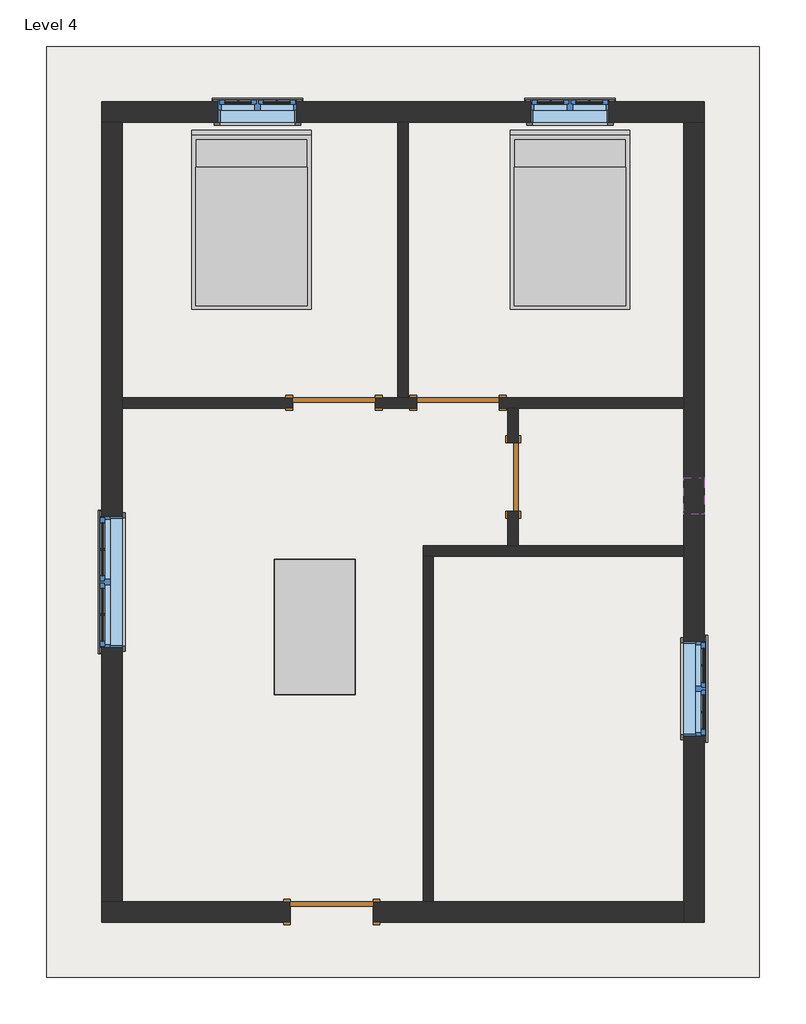
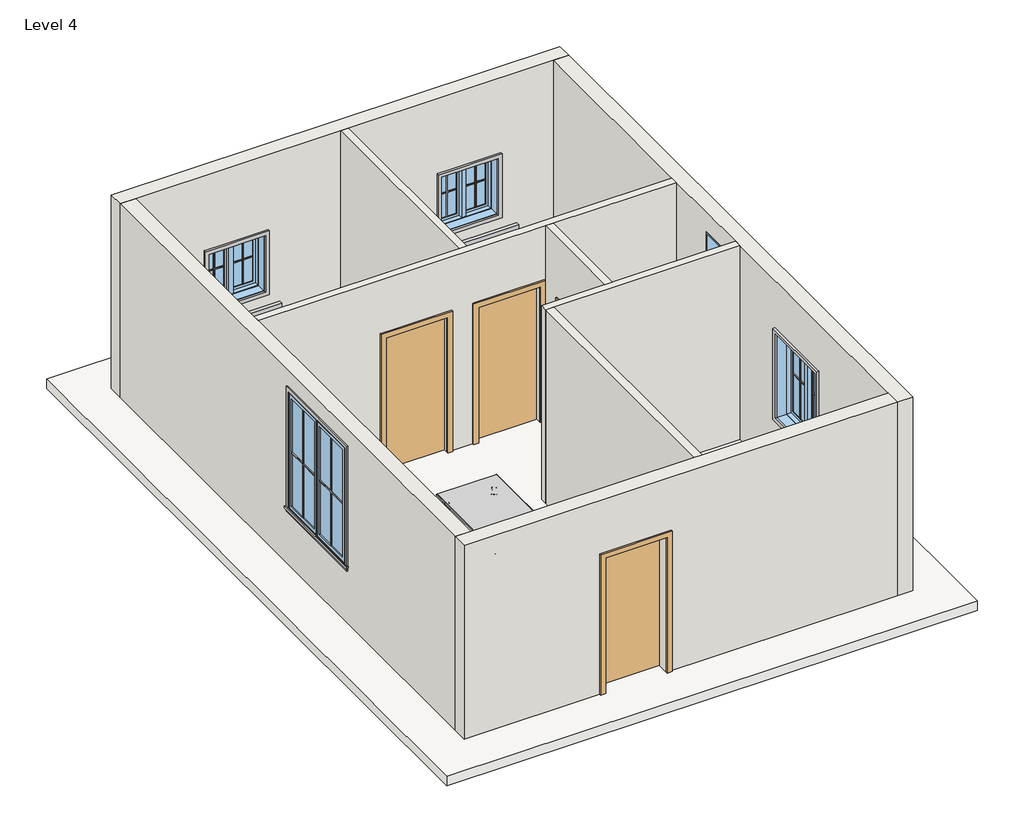
# One storey, incomplete: 16 proxies, 9 walls, 5 windows, 4 doors, 3 furniture elements, 1 roof.
"""IFC4 building model written with IfcOpenShell, lengths in millimetres."""

from ifc_helpers import new_model, si_unit, frame, origin, place, context, project, spatial, polyline, outline, extrude, faceted_brep, transform, mapped, element, save
from components import muntin_pattern_2x2_muntin_pattern_2x2_b3fe6957, muntin_pattern_2x2_muntin_pattern_2x2_3e0ecaf2, muntin_pattern_2x2_muntin_pattern_2x2_bff912c5, muntin_pattern_2x2_muntin_pattern_2x2_c2194282, muntin_pattern_2x2_muntin_pattern_2x2_88bf7f41, muntin_pattern_2x2_muntin_pattern_2x2_3dfd0a47, trim_window_exterior_flat_with_sill_41619996, trim_window_exterior_flat_with_sill_e04b3088, trim_window_exterior_flat_with_sill_4930676f, trim_window_interior_flat_picture_frame_51c85655, trim_window_interior_flat_picture_frame_2a7685fe, trim_window_interior_flat_picture_frame_dd064338, door_f2b275c1, door_e5f9f3c4, door_305aa2a5, door_0ca8825f, bed_17739_bed_17739_15c61121, dining_table_14755_dining_table_14755_d89cb775, window_aa618e30, window_339605e1, window_c95ebb39, window_9ac97e1a

model = new_model("IFC4")

# Units and contexts
model_context = context("Model", 3, world=origin())
ifc_project = project(units=[si_unit("LENGTHUNIT", "METRE", prefix="MILLI")], contexts=[model_context])

# Site, building, storey
site = spatial("IfcSite", under=ifc_project)
building = spatial("IfcBuilding", under=site)
storey = spatial("IfcBuildingStorey", under=building, Name="Level 4", Elevation=6400.8)

# Proxies
placement = place(None, origin())
muntin_pattern_2x2_muntin_pattern_2x2_shape = muntin_pattern_2x2_muntin_pattern_2x2_b3fe6957(model_context)
element("IfcBuildingElementProxy", 1, Name="Muntin Pattern_2x2 : Muntin Pattern_2x2", ObjectType="Muntin Pattern_2x2 : Muntin Pattern_2x2", at=placement, inside=storey, context=model_context, shape_type="MappedRepresentation", body=[
    mapped(muntin_pattern_2x2_muntin_pattern_2x2_shape, transform((-3079.2790084, 5068.9185985, 7385.05), x_axis=(1.0, 0.0, 0.0), y_axis=(0.0, 1.0, 0.0), z_axis=(0.0, 0.0, 1.0))),
])
element("IfcBuildingElementProxy", 2, Name="Muntin Pattern_2x2 : Muntin Pattern_2x2", ObjectType="Muntin Pattern_2x2 : Muntin Pattern_2x2", at=placement, inside=storey, context=model_context, shape_type="MappedRepresentation", body=[
    mapped(muntin_pattern_2x2_muntin_pattern_2x2_shape, transform((378.2959916, 5068.9185985, 7385.05), x_axis=(1.0, 0.0, 0.0), y_axis=(0.0, 1.0, 0.0), z_axis=(0.0, 0.0, 1.0))),
])
muntin_pattern_2x2_muntin_pattern_2x2_2_shape = muntin_pattern_2x2_muntin_pattern_2x2_3e0ecaf2(model_context)
element("IfcBuildingElementProxy", 3, Name="Muntin Pattern_2x2 : Muntin Pattern_2x2", ObjectType="Muntin Pattern_2x2 : Muntin Pattern_2x2", at=placement, inside=storey, context=model_context, shape_type="MappedRepresentation", body=[
    mapped(muntin_pattern_2x2_muntin_pattern_2x2_2_shape, transform((-2650.6540084, 5068.9185985, 7385.05), x_axis=(-1.0, 0.0, 0.0), y_axis=(0.0, -1.0, 0.0), z_axis=(0.0, 0.0, 1.0))),
])
element("IfcBuildingElementProxy", 4, Name="Muntin Pattern_2x2 : Muntin Pattern_2x2", ObjectType="Muntin Pattern_2x2 : Muntin Pattern_2x2", at=placement, inside=storey, context=model_context, shape_type="MappedRepresentation", body=[
    mapped(muntin_pattern_2x2_muntin_pattern_2x2_2_shape, transform((806.9209916, 5068.9185985, 7385.05), x_axis=(-1.0, 0.0, 0.0), y_axis=(0.0, -1.0, 0.0), z_axis=(0.0, 0.0, 1.0))),
])
muntin_pattern_2x2_muntin_pattern_2x2_3_shape = muntin_pattern_2x2_muntin_pattern_2x2_bff912c5(model_context)
element("IfcBuildingElementProxy", 5, Name="Muntin Pattern_2x2 : Muntin Pattern_2x2", ObjectType="Muntin Pattern_2x2 : Muntin Pattern_2x2", at=placement, inside=storey, context=model_context, shape_type="MappedRepresentation", body=[
    mapped(muntin_pattern_2x2_muntin_pattern_2x2_3_shape, transform((-4579.4665084, -596.8689015, 7385.05), x_axis=(0.0, 1.0, 0.0), y_axis=(-1.0, 0.0, 0.0), z_axis=(0.0, 0.0, 1.0))),
])
muntin_pattern_2x2_muntin_pattern_2x2_4_shape = muntin_pattern_2x2_muntin_pattern_2x2_c2194282(model_context)
element("IfcBuildingElementProxy", 6, Name="Muntin Pattern_2x2 : Muntin Pattern_2x2", ObjectType="Muntin Pattern_2x2 : Muntin Pattern_2x2", at=placement, inside=storey, context=model_context, shape_type="MappedRepresentation", body=[
    mapped(muntin_pattern_2x2_muntin_pattern_2x2_4_shape, transform((-4579.4665084, 123.8560985, 7385.05), x_axis=(0.0, -1.0, 0.0), y_axis=(1.0, 0.0, 0.0), z_axis=(0.0, 0.0, 1.0))),
])
muntin_pattern_2x2_muntin_pattern_2x2_5_shape = muntin_pattern_2x2_muntin_pattern_2x2_88bf7f41(model_context)
element("IfcBuildingElementProxy", 7, Name="Muntin Pattern_2x2 : Muntin Pattern_2x2", ObjectType="Muntin Pattern_2x2 : Muntin Pattern_2x2", at=placement, inside=storey, context=model_context, shape_type="MappedRepresentation", body=[
    mapped(muntin_pattern_2x2_muntin_pattern_2x2_5_shape, transform((2068.9834916, -1158.8439015, 7385.05), x_axis=(0.0, -1.0, 0.0), y_axis=(1.0, 0.0, 0.0), z_axis=(0.0, 0.0, 1.0))),
])
muntin_pattern_2x2_muntin_pattern_2x2_6_shape = muntin_pattern_2x2_muntin_pattern_2x2_3dfd0a47(model_context)
element("IfcBuildingElementProxy", 8, Name="Muntin Pattern_2x2 : Muntin Pattern_2x2", ObjectType="Muntin Pattern_2x2 : Muntin Pattern_2x2", at=placement, inside=storey, context=model_context, shape_type="MappedRepresentation", body=[
    mapped(muntin_pattern_2x2_muntin_pattern_2x2_6_shape, transform((2068.9834916, -1676.3689015, 7385.05), x_axis=(0.0, 1.0, 0.0), y_axis=(-1.0, 0.0, 0.0), z_axis=(0.0, 0.0, 1.0))),
])
trim_window_exterior_flat_with_sill_shape = trim_window_exterior_flat_with_sill_41619996(model_context)
element("IfcBuildingElementProxy", 9, Name="Trim-Window-Exterior-Flat : with Sill", ObjectType="Trim-Window-Exterior-Flat : with Sill", at=placement, inside=storey, context=model_context, shape_type="MappedRepresentation", body=[
    mapped(trim_window_exterior_flat_with_sill_shape, transform((-2864.9665084, 5078.4435985, 8229.6), x_axis=(-1.0, 0.0, 0.0), y_axis=(0.0, 0.0, 1.0), z_axis=(0.0, 1.0, 0.0))),
])
element("IfcBuildingElementProxy", 10, Name="Trim-Window-Exterior-Flat : with Sill", ObjectType="Trim-Window-Exterior-Flat : with Sill", at=placement, inside=storey, context=model_context, shape_type="MappedRepresentation", body=[
    mapped(trim_window_exterior_flat_with_sill_shape, transform((592.6084916, 5078.4435985, 8229.6), x_axis=(-1.0, 0.0, 0.0), y_axis=(0.0, 0.0, 1.0), z_axis=(0.0, 1.0, 0.0))),
])
trim_window_exterior_flat_with_sill_2_shape = trim_window_exterior_flat_with_sill_e04b3088(model_context)
element("IfcBuildingElementProxy", 11, Name="Trim-Window-Exterior-Flat : with Sill", ObjectType="Trim-Window-Exterior-Flat : with Sill", at=placement, inside=storey, context=model_context, shape_type="MappedRepresentation", body=[
    mapped(trim_window_exterior_flat_with_sill_2_shape, transform((-4588.9915084, -236.5064015, 9144.0), x_axis=(0.0, -1.0, 0.0), y_axis=(0.0, 0.0, 1.0), z_axis=(-1.0, 0.0, 0.0))),
])
trim_window_exterior_flat_with_sill_3_shape = trim_window_exterior_flat_with_sill_4930676f(model_context)
element("IfcBuildingElementProxy", 12, Name="Trim-Window-Exterior-Flat : with Sill", ObjectType="Trim-Window-Exterior-Flat : with Sill", at=placement, inside=storey, context=model_context, shape_type="MappedRepresentation", body=[
    mapped(trim_window_exterior_flat_with_sill_3_shape, transform((2078.5084916, -1417.6064015, 8661.4), x_axis=(0.0, 1.0, 0.0), y_axis=(0.0, 0.0, 1.0), z_axis=(1.0, 0.0, 0.0))),
])
trim_window_interior_flat_picture_frame_shape = trim_window_interior_flat_picture_frame_51c85655(model_context)
element("IfcBuildingElementProxy", 13, Name="Trim-Window-Interior-Flat : Picture Frame", ObjectType="Trim-Window-Interior-Flat : Picture Frame", at=placement, inside=storey, context=model_context, shape_type="MappedRepresentation", body=[
    mapped(trim_window_interior_flat_picture_frame_shape, transform((-2864.9665084, 4849.8435985, 8229.6), x_axis=(1.0, 0.0, 0.0), y_axis=(0.0, 0.0, 1.0), z_axis=(0.0, -1.0, 0.0))),
])
element("IfcBuildingElementProxy", 14, Name="Trim-Window-Interior-Flat : Picture Frame", ObjectType="Trim-Window-Interior-Flat : Picture Frame", at=placement, inside=storey, context=model_context, shape_type="MappedRepresentation", body=[
    mapped(trim_window_interior_flat_picture_frame_shape, transform((592.6084916, 4849.8435985, 8229.6), x_axis=(1.0, 0.0, 0.0), y_axis=(0.0, 0.0, 1.0), z_axis=(0.0, -1.0, 0.0))),
])
trim_window_interior_flat_picture_frame_2_shape = trim_window_interior_flat_picture_frame_2a7685fe(model_context)
element("IfcBuildingElementProxy", 15, Name="Trim-Window-Interior-Flat : Picture Frame", ObjectType="Trim-Window-Interior-Flat : Picture Frame", at=placement, inside=storey, context=model_context, shape_type="MappedRepresentation", body=[
    mapped(trim_window_interior_flat_picture_frame_2_shape, transform((-4360.3915084, -236.5064015, 9144.0), x_axis=(0.0, 1.0, 0.0), y_axis=(0.0, 0.0, 1.0), z_axis=(1.0, 0.0, 0.0))),
])
trim_window_interior_flat_picture_frame_3_shape = trim_window_interior_flat_picture_frame_dd064338(model_context)
element("IfcBuildingElementProxy", 16, Name="Trim-Window-Interior-Flat : Picture Frame", ObjectType="Trim-Window-Interior-Flat : Picture Frame", at=placement, inside=storey, context=model_context, shape_type="MappedRepresentation", body=[
    mapped(trim_window_interior_flat_picture_frame_3_shape, transform((1849.9084916, -1417.6064015, 8661.4), x_axis=(0.0, -1.0, 0.0), y_axis=(0.0, 0.0, 1.0), z_axis=(-1.0, 0.0, 0.0))),
])

# Doors
door_shape = door_f2b275c1(model_context)
element("IfcDoor", 17, ObjectType="Single-Flush : 30\" x 80\"", at=placement, inside=storey, context=model_context, shape_type="MappedRepresentation", body=[
    mapped(door_shape, transform((-36.0415084, 925.5435985, 6400.8), x_axis=(0.0, 1.0, 0.0), y_axis=(-1.0, 0.0, 0.0), z_axis=(0.0, 0.0, 1.0))),
])
door_2_shape = door_e5f9f3c4(model_context)
element("IfcDoor", 18, ObjectType="Single-Flush : 36\" x 84\"", at=placement, inside=storey, context=model_context, shape_type="MappedRepresentation", body=[
    mapped(door_2_shape, transform((-2017.2415084, 1744.6935985, 6400.8), x_axis=(1.0, 0.0, 0.0), y_axis=(0.0, 1.0, 0.0), z_axis=(0.0, 0.0, 1.0))),
])
door_3_shape = door_305aa2a5(model_context)
element("IfcDoor", 19, ObjectType="Single-Flush : 36\" x 84\"", at=placement, inside=storey, context=model_context, shape_type="MappedRepresentation", body=[
    mapped(door_3_shape, transform((-645.6415084, 1744.6935985, 6400.8), x_axis=(-1.0, 0.0, 0.0), y_axis=(0.0, -1.0, 0.0), z_axis=(0.0, 0.0, 1.0))),
])
door_4_shape = door_0ca8825f(model_context)
element("IfcDoor", 20, ObjectType="Single-Flush : 36\" x 84\"", at=placement, inside=storey, context=model_context, shape_type="MappedRepresentation", body=[
    mapped(door_4_shape, transform((-2042.6415084, -3887.7564015, 6400.8), x_axis=(1.0, 0.0, 0.0), y_axis=(0.0, 1.0, 0.0), z_axis=(0.0, 0.0, 1.0))),
])

# Furniture
bed_17739_bed_17739_shape = bed_17739_bed_17739_15c61121(model_context)
element("IfcFurniture", 21, ObjectType="Bed_17739 : Bed_17739", at=placement, inside=storey, context=model_context, shape_type="MappedRepresentation", body=[
    mapped(bed_17739_bed_17739_shape, transform((-2931.6415084, 3744.9435985, 6400.8), x_axis=(1.0, 0.0, 0.0), y_axis=(0.0, 1.0, 0.0), z_axis=(0.0, 0.0, 1.0))),
])
element("IfcFurniture", 22, ObjectType="Bed_17739 : Bed_17739", at=placement, inside=storey, context=model_context, shape_type="MappedRepresentation", body=[
    mapped(bed_17739_bed_17739_shape, transform((592.6084916, 3744.9435985, 6400.8), x_axis=(1.0, 0.0, 0.0), y_axis=(0.0, 1.0, 0.0), z_axis=(0.0, 0.0, 1.0))),
])
dining_table_14755_dining_table_14755_shape = dining_table_14755_dining_table_14755_d89cb775(model_context)
element("IfcFurniture", 23, ObjectType="Dining_table_14755 : Dining_table_14755", at=placement, inside=storey, context=model_context, shape_type="MappedRepresentation", body=[
    mapped(dining_table_14755_dining_table_14755_shape, transform((-1781.6222109, -1485.4350296, 6400.8), x_axis=(0.0, 1.0, 0.0), y_axis=(-1.0, 0.0, 0.0), z_axis=(0.0, 0.0, 1.0))),
])

# Roof
element("IfcRoof", 24, ObjectType="Generic - 12\"", at=placement, inside=storey, context=model_context, shape_type="SweptSolid", body=[
    extrude(outline(polyline([(-5198.5915084, 5688.0435985), (2688.1084916, 5688.0435985), (2688.1084916, -4611.6564015), (-5198.5915084, -4611.6564015), (-5198.5915084, 5688.0435985)])), frame((0.0, 0.0, 6248.4), z_axis=(0.0, 0.0, 1.0), x_axis=(1.0, 0.0, 0.0)), (0.0, 0.0, 1.0), 152.4),
])

# Walls
element("IfcWall", 25, ObjectType="WALL4.5\"", at=placement, inside=storey, context=model_context, shape_type="Brep", body=[
    faceted_brep([(-1560.0415084, 1687.5435985, 6400.8), (-1102.8415084, 1687.5435985, 6400.8), (-1102.8415084, 1687.5435985, 8534.4), (-188.4415084, 1687.5435985, 8534.4), (-188.4415084, 1687.5435985, 6400.8), (-93.1915084, 1687.5435985, 6400.8), (21.1084916, 1687.5435985, 6400.8), (1849.9084916, 1687.5435985, 6400.8), (1849.9084916, 1687.5435985, 9448.8), (21.1084916, 1687.5435985, 9448.8), (-93.1915084, 1687.5435985, 9448.8), (-4360.3915084, 1687.5435985, 9448.8), (-4360.3915084, 1687.5435985, 6400.8), (-2474.4415084, 1687.5435985, 6400.8), (-2474.4415084, 1687.5435985, 8534.4), (-1560.0415084, 1687.5435985, 8534.4), (-1102.8415084, 1801.8435985, 8534.4), (-1102.8415084, 1801.8435985, 6400.8), (-1198.0915084, 1801.8435985, 6400.8), (-1312.3915084, 1801.8435985, 6400.8), (-1560.0415084, 1801.8435985, 6400.8), (-1560.0415084, 1801.8435985, 8534.4), (-2474.4415084, 1801.8435985, 8534.4), (-2474.4415084, 1801.8435985, 6400.8), (-4360.3915084, 1801.8435985, 6400.8), (-4360.3915084, 1801.8435985, 9448.8), (-1312.3915084, 1801.8435985, 9448.8), (-1198.0915084, 1801.8435985, 9448.8), (1849.9084916, 1801.8435985, 9448.8), (1849.9084916, 1801.8435985, 6400.8), (-188.4415084, 1801.8435985, 6400.8), (-188.4415084, 1801.8435985, 8534.4)], [[[0, 1, 2, 3, 4, 5, 6, 7, 8, 9, 10, 11, 12, 13, 14, 15]], [[16, 17, 18, 19, 20, 21, 22, 23, 24, 25, 26, 27, 28, 29, 30, 31]], [[13, 12, 24, 23]], [[30, 29, 7, 6, 5, 4]], [[20, 19, 18, 17, 1, 0]], [[8, 7, 29, 28]], [[12, 11, 25, 24]], [[21, 20, 0, 15]], [[22, 21, 15, 14]], [[23, 22, 14, 13]], [[2, 1, 17, 16]], [[3, 2, 16, 31]], [[4, 3, 31, 30]], [[11, 10, 9, 8, 28, 27, 26, 25]]]),
])
element("IfcWall", 26, ObjectType="WALL4.5\"", at=placement, inside=storey, context=model_context, shape_type="SweptSolid", body=[
    extrude(outline(polyline([(-1312.3915084, 1801.8435985), (-1312.3915084, 4849.8435985), (-1198.0915084, 4849.8435985), (-1198.0915084, 1801.8435985), (-1312.3915084, 1801.8435985)])), frame((0.0, 0.0, 6400.8), z_axis=(0.0, 0.0, 1.0), x_axis=(1.0, 0.0, 0.0)), (0.0, 0.0, 1.0), 3048.0),
])
element("IfcWall", 27, ObjectType="WALL4.5\"", at=placement, inside=storey, context=model_context, shape_type="SweptSolid", body=[
    extrude(outline(polyline([(1687.5435985, 6400.8), (1306.5435985, 6400.8), (1306.5435985, 8432.8), (544.5435985, 8432.8), (544.5435985, 6400.8), (163.5435985, 6400.8), (163.5435985, 9448.8), (1687.5435985, 9448.8), (1687.5435985, 6400.8)])), frame((-93.1915084, 0.0, 0.0), z_axis=(1.0, 0.0, 0.0), x_axis=(0.0, 1.0, 0.0)), (0.0, 0.0, 1.0), 114.3),
])
element("IfcWall", 28, ObjectType="WALL4.5\"", at=placement, inside=storey, context=model_context, shape_type="Brep", body=[
    faceted_brep([(1849.9084916, 163.5435985, 6400.8), (21.1084916, 163.5435985, 6400.8), (-93.1915084, 163.5435985, 6400.8), (-1032.9915084, 163.5435985, 6400.8), (-1032.9915084, 163.5435985, 9448.8), (-93.1915084, 163.5435985, 9448.8), (21.1084916, 163.5435985, 9448.8), (1849.9084916, 163.5435985, 9448.8), (1849.9084916, 49.2435985, 6400.8), (1849.9084916, 49.2435985, 9448.8), (-918.6915084, 49.2435985, 9448.8), (-1032.9915084, 49.2435985, 9448.8), (-1032.9915084, 49.2435985, 6400.8), (-918.6915084, 49.2435985, 6400.8)], [[[0, 1, 2, 3, 4, 5, 6, 7]], [[8, 9, 10, 11, 12, 13]], [[3, 2, 1, 0, 8, 13, 12]], [[0, 7, 9, 8]], [[4, 3, 12, 11]], [[7, 6, 5, 4, 11, 10, 9]]]),
])
element("IfcWall", 29, ObjectType="WALL4.5\"", at=placement, inside=storey, context=model_context, shape_type="SweptSolid", body=[
    extrude(outline(polyline([(-1032.9915084, -3773.4564015), (-1032.9915084, 49.2435985), (-918.6915084, 49.2435985), (-918.6915084, -3773.4564015), (-1032.9915084, -3773.4564015)])), frame((0.0, 0.0, 6400.8), z_axis=(0.0, 0.0, 1.0), x_axis=(1.0, 0.0, 0.0)), (0.0, 0.0, 1.0), 3048.0),
])
element("IfcWall", 30, ObjectType="WALL9\"", at=placement, inside=storey, context=model_context, shape_type="Brep", body=[
    faceted_brep([(-4588.9915084, 4849.8435985, 6400.8), (-4360.3915084, 4849.8435985, 6400.8), (-1312.3915084, 4849.8435985, 6400.8), (-1198.0915084, 4849.8435985, 6400.8), (1849.9084916, 4849.8435985, 6400.8), (2078.5084916, 4849.8435985, 6400.8), (2078.5084916, 4849.8435985, 9448.8), (1849.9084916, 4849.8435985, 9448.8), (-1198.0915084, 4849.8435985, 9448.8), (-1312.3915084, 4849.8435985, 9448.8), (-4360.3915084, 4849.8435985, 9448.8), (-4588.9915084, 4849.8435985, 9448.8), (-2433.1665084, 4849.8435985, 8229.6), (-2433.1665084, 4849.8435985, 7315.2), (-3296.7665084, 4849.8435985, 7315.2), (-3296.7665084, 4849.8435985, 8229.6), (1024.4084916, 4849.8435985, 8229.6), (1024.4084916, 4849.8435985, 7315.2), (160.8084916, 4849.8435985, 7315.2), (160.8084916, 4849.8435985, 8229.6), (-4588.9915084, 5078.4435985, 6400.8), (-4588.9915084, 5078.4435985, 9448.8), (2078.5084916, 5078.4435985, 9448.8), (2078.5084916, 5078.4435985, 6400.8), (-2433.1665084, 5078.4435985, 8229.6), (-3296.7665084, 5078.4435985, 8229.6), (-3296.7665084, 5078.4435985, 7315.2), (-2433.1665084, 5078.4435985, 7315.2), (1024.4084916, 5078.4435985, 8229.6), (160.8084916, 5078.4435985, 8229.6), (160.8084916, 5078.4435985, 7315.2), (1024.4084916, 5078.4435985, 7315.2)], [[[0, 1, 2, 3, 4, 5, 6, 7, 8, 9, 10, 11], [12, 13, 14, 15], [16, 17, 18, 19]], [[20, 21, 22, 23], [24, 25, 26, 27], [28, 29, 30, 31]], [[5, 4, 3, 2, 1, 0, 20, 23]], [[6, 5, 23, 22]], [[0, 11, 21, 20]], [[13, 12, 24, 27]], [[14, 13, 27, 26]], [[15, 14, 26, 25]], [[12, 15, 25, 24]], [[17, 16, 28, 31]], [[18, 17, 31, 30]], [[19, 18, 30, 29]], [[16, 19, 29, 28]], [[11, 10, 9, 8, 7, 6, 22, 21]]]),
])
element("IfcWall", 31, ObjectType="WALL9\"", at=placement, inside=storey, context=model_context, shape_type="Brep", body=[
    faceted_brep([(1849.9084916, 4849.8435985, 6400.8), (1849.9084916, 1801.8435985, 6400.8), (1849.9084916, 1687.5435985, 6400.8), (1849.9084916, 163.5435985, 6400.8), (1849.9084916, 49.2435985, 6400.8), (1849.9084916, -3773.4564015, 6400.8), (1849.9084916, -4002.0564015, 6400.8), (1849.9084916, -4002.0564015, 9448.8), (1849.9084916, -3773.4564015, 9448.8), (1849.9084916, 49.2435985, 9448.8), (1849.9084916, 163.5435985, 9448.8), (1849.9084916, 1687.5435985, 9448.8), (1849.9084916, 1801.8435985, 9448.8), (1849.9084916, 4849.8435985, 9448.8), (1849.9084916, -1938.3064015, 8661.4), (1849.9084916, -1938.3064015, 7315.2), (1849.9084916, -896.9064015, 7315.2), (1849.9084916, -896.9064015, 8661.4), (1849.9084916, 512.7935985, 9144.0), (1849.9084916, 512.7935985, 8534.4), (1849.9084916, 919.1935985, 8534.4), (1849.9084916, 919.1935985, 9144.0), (2078.5084916, 4849.8435985, 6400.8), (2078.5084916, 4849.8435985, 9448.8), (2078.5084916, -4002.0564015, 9448.8), (2078.5084916, -4002.0564015, 6400.8), (2078.5084916, -1938.3064015, 8661.4), (2078.5084916, -896.9064015, 8661.4), (2078.5084916, -896.9064015, 7315.2), (2078.5084916, -1938.3064015, 7315.2), (2078.5084916, 512.7935985, 9144.0), (2078.5084916, 919.1935985, 9144.0), (2078.5084916, 919.1935985, 8534.4), (2078.5084916, 512.7935985, 8534.4)], [[[0, 1, 2, 3, 4, 5, 6, 7, 8, 9, 10, 11, 12, 13], [14, 15, 16, 17], [18, 19, 20, 21]], [[22, 23, 24, 25], [26, 27, 28, 29], [30, 31, 32, 33]], [[6, 5, 4, 3, 2, 1, 0, 22, 25]], [[0, 13, 23, 22]], [[7, 6, 25, 24]], [[15, 14, 26, 29]], [[16, 15, 29, 28]], [[17, 16, 28, 27]], [[14, 17, 27, 26]], [[19, 18, 30, 33]], [[20, 19, 33, 32]], [[21, 20, 32, 31]], [[18, 21, 31, 30]], [[13, 12, 11, 10, 9, 8, 7, 24, 23]]]),
])
element("IfcWall", 32, ObjectType="WALL9\"", at=placement, inside=storey, context=model_context, shape_type="Brep", body=[
    faceted_brep([(1849.9084916, -3773.4564015, 6400.8), (-918.6915084, -3773.4564015, 6400.8), (-1032.9915084, -3773.4564015, 6400.8), (-1585.4415084, -3773.4564015, 6400.8), (-1585.4415084, -3773.4564015, 8534.4), (-2499.8415084, -3773.4564015, 8534.4), (-2499.8415084, -3773.4564015, 6400.8), (-4360.3915084, -3773.4564015, 6400.8), (-4588.9915084, -3773.4564015, 6400.8), (-4588.9915084, -3773.4564015, 9448.8), (-4360.3915084, -3773.4564015, 9448.8), (-1032.9915084, -3773.4564015, 9448.8), (-918.6915084, -3773.4564015, 9448.8), (1849.9084916, -3773.4564015, 9448.8), (-1585.4415084, -4002.0564015, 8534.4), (-1585.4415084, -4002.0564015, 6400.8), (1849.9084916, -4002.0564015, 6400.8), (1849.9084916, -4002.0564015, 9448.8), (-4588.9915084, -4002.0564015, 9448.8), (-4588.9915084, -4002.0564015, 6400.8), (-2499.8415084, -4002.0564015, 6400.8), (-2499.8415084, -4002.0564015, 8534.4)], [[[0, 1, 2, 3, 4, 5, 6, 7, 8, 9, 10, 11, 12, 13]], [[14, 15, 16, 17, 18, 19, 20, 21]], [[20, 19, 8, 7, 6]], [[16, 15, 3, 2, 1, 0]], [[0, 13, 17, 16]], [[9, 8, 19, 18]], [[4, 3, 15, 14]], [[5, 4, 14, 21]], [[6, 5, 21, 20]], [[13, 12, 11, 10, 9, 18, 17]]]),
])
element("IfcWall", 33, ObjectType="WALL9\"", at=placement, inside=storey, context=model_context, shape_type="Brep", body=[
    faceted_brep([(-4360.3915084, -3773.4564015, 6400.8), (-4360.3915084, 1687.5435985, 6400.8), (-4360.3915084, 1801.8435985, 6400.8), (-4360.3915084, 4849.8435985, 6400.8), (-4360.3915084, 4849.8435985, 9448.8), (-4360.3915084, 1801.8435985, 9448.8), (-4360.3915084, 1687.5435985, 9448.8), (-4360.3915084, -3773.4564015, 9448.8), (-4360.3915084, 487.3935985, 9144.0), (-4360.3915084, 487.3935985, 7315.2), (-4360.3915084, -960.4064015, 7315.2), (-4360.3915084, -960.4064015, 9144.0), (-4588.9915084, -3773.4564015, 6400.8), (-4588.9915084, -3773.4564015, 9448.8), (-4588.9915084, 4849.8435985, 9448.8), (-4588.9915084, 4849.8435985, 6400.8), (-4588.9915084, 487.3935985, 9144.0), (-4588.9915084, -960.4064015, 9144.0), (-4588.9915084, -960.4064015, 7315.2), (-4588.9915084, 487.3935985, 7315.2)], [[[0, 1, 2, 3, 4, 5, 6, 7], [8, 9, 10, 11]], [[12, 13, 14, 15], [16, 17, 18, 19]], [[3, 2, 1, 0, 12, 15]], [[0, 7, 13, 12]], [[4, 3, 15, 14]], [[9, 8, 16, 19]], [[10, 9, 19, 18]], [[11, 10, 18, 17]], [[8, 11, 17, 16]], [[7, 6, 5, 4, 14, 13]]]),
])

# Windows
window_shape = window_aa618e30(model_context)
element("IfcWindow", 34, ObjectType="Fixed : 16\" x 24\"", at=placement, inside=storey, context=model_context, shape_type="MappedRepresentation", body=[
    mapped(window_shape, transform((1964.2084916, 677.8935985, 7620.0), x_axis=(0.0, -1.0, 0.0), y_axis=(1.0, 0.0, 0.0), z_axis=(0.0, 0.0, 1.0))),
])
window_2_shape = window_339605e1(model_context)
element("IfcWindow", 35, ObjectType="Window-Casement-Double : 34\" x 36\"", at=placement, inside=storey, context=model_context, shape_type="MappedRepresentation", body=[
    mapped(window_2_shape, transform((-2864.9665084, 4964.1435985, 6400.8), x_axis=(1.0, 0.0, 0.0), y_axis=(0.0, 1.0, 0.0), z_axis=(0.0, 0.0, 1.0))),
])
element("IfcWindow", 36, ObjectType="Window-Casement-Double : 34\" x 36\"", at=placement, inside=storey, context=model_context, shape_type="MappedRepresentation", body=[
    mapped(window_2_shape, transform((592.6084916, 4964.1435985, 6400.8), x_axis=(1.0, 0.0, 0.0), y_axis=(0.0, 1.0, 0.0), z_axis=(0.0, 0.0, 1.0))),
])
window_3_shape = window_c95ebb39(model_context)
element("IfcWindow", 37, ObjectType="Window-Casement-Double : 41\" x 53\"", at=placement, inside=storey, context=model_context, shape_type="MappedRepresentation", body=[
    mapped(window_3_shape, transform((1964.2084916, -1417.6064015, 6400.8), x_axis=(0.0, -1.0, 0.0), y_axis=(1.0, 0.0, 0.0), z_axis=(0.0, 0.0, 1.0))),
])
window_4_shape = window_9ac97e1a(model_context)
element("IfcWindow", 38, ObjectType="Window-Casement-Double : 57\" x 72\"", at=placement, inside=storey, context=model_context, shape_type="MappedRepresentation", body=[
    mapped(window_4_shape, transform((-4474.6915084, -236.5064015, 6400.8), x_axis=(0.0, 1.0, 0.0), y_axis=(-1.0, 0.0, 0.0), z_axis=(0.0, 0.0, 1.0))),
])

save(model, "model.ifc")

# Revit data of these elements
# Type "Muntin Pattern_2x2 : Muntin Pattern_2x2"
#   Width [instance default] = 4' - 0"
#   Thickness = 0' - 0 1/2"
#   Height [instance default] = 4' - 0"
#   Distance = 0' - 0 3/4"
#   Interior Material [instance default] = none
#   Exterior Material [instance default] = none
#   Default Elevation = 0
# Type "Trim-Window-Exterior-Flat : with Sill"
#   Trim Width = 0' - 2 1/4"
#   Trim Thickness_Picture Frame = 0' - 1 1/4"
#   Trim Thickness_with Sill = 0' - 0 3/4"
#   Sill Thickness = 0' - 1 1/4"
#   Opening Width [instance default] = 2' - 0"
#   Opening Height [instance default] = 3' - 0"
#   Default Elevation = 4' - 0"
#   Sill = yes
#   Picture Frame = no
#   Trim Material [instance default] = none
# Type "Trim-Window-Interior-Flat : Picture Frame"
#   Trim Thickness_Picture Frame = 0' - 1 1/4"
#   Trim Width = 0' - 2 1/4"
#   Trim Thickness_with Sill = 0' - 0 3/4"
#   Sill Thickness = 0' - 1 1/4"
#   Opening Width [instance default] = 2' - 0"
#   Opening Height [instance default] = 3' - 0"
#   Default Elevation = 4' - 0"
#   Sill = no
#   Picture Frame = yes
#   Trim Material [instance default] = none
# Type "Single-Flush : 30\" x 80\""
#   Type Mark = "5"
#   Construction Type Id = "MDOOR"
#   Assembly Code = "C1020"
#   Analytic Construction = "Metal"
#   Thickness = 0' - 2"
#   Heat Transfer Coefficient (U) = 0.651978 BTU/(h·ft²·°F)
#   Height = 6' - 8"
#   Trim Projection Ext = 0' - 1"
#   Trim Projection Int = 0' - 1"
#   Trim Width = 0' - 3"
#   Width = 2' - 6"
#   Define Thermal Properties by = 1
#   Define Thermal Properties by = 1
#   Door Material = Door - Panel
#   Frame Material = Door - Frame
#   Visual Light Transmittance = 0
#   Solar Heat Gain Coefficient = 0
#   Function = (empty or 0)
#   Wall Closure = (empty or 0)
# Type "Single-Flush : 36\" x 84\""
#   Type Mark = "1"
#   Construction Type Id = "MDOOR"
#   Assembly Code = "C1020"
#   Analytic Construction = "Metal"
#   Thickness = 0' - 2"
#   Heat Transfer Coefficient (U) = 0.651978 BTU/(h·ft²·°F)
#   Height = 7' - 0"
#   Trim Projection Ext = 0' - 1"
#   Trim Projection Int = 0' - 1"
#   Trim Width = 0' - 3"
#   Width = 3' - 0"
#   Define Thermal Properties by = 1
#   Define Thermal Properties by = 1
#   Door Material = Door - Panel
#   Frame Material = Door - Frame
#   Visual Light Transmittance = 0
#   Solar Heat Gain Coefficient = 0
#   Function = (empty or 0)
#   Wall Closure = (empty or 0)
# Type "Bed_17739 : Bed_17739"
#   Default Elevation = 0
# Type "Dining_table_14755 : Dining_table_14755"
#   Lengte [instance default] = 4' - 11.05512"
#   Breedte [instance default] = 2' - 11.43307"
#   Tafelblad = none
#   Poten = none
#   Default Elevation = 0
# Type "Generic - 12\""
#   Assembly Code = "B1020"
#   Layers, outside or top first: 0' - 6" no material (function 1)
# Type "WALL4.5\""
#   Assembly Code = "B2010"
#   Layers, outside or top first: 0' - 4 1/2" no material (function 1)
# Type "WALL9\""
#   Assembly Code = "B2010"
#   Layers, outside or top first: 0' - 9" no material (function 1)
# Type "Fixed : 16\" x 24\""
#   Type Mark = "4"
#   Construction Type Id = "GSP4R"
#   Assembly Code = "B2020100"
#   Analytic Construction = "1/8 in Pilkington single glazing"
#   Visual Light Transmittance = 0.9
#   Solar Heat Gain Coefficient = 0.78
#   Heat Transfer Coefficient (U) = 0.6496 BTU/(h·ft²·°F)
#   Height = 2' - 0"
#   Default Sill Height = 3' - 0"
#   Width = 1' - 4"
#   Window Inset = 0' - 0 3/4"
#   Define Thermal Properties by = 1
#   Define Thermal Properties by = 1
#   Glass Pane Material = Glass
#   Sash Material = Sash
#   Wall Closure = (empty or 0)
# Type "Window-Casement-Double : 34\" x 36\""
#   Type Mark = "14"
#   Fire Rating = "0.5h"
#   Assembly Code = "B2020100"
#   Analytic Construction = "Double glazing - domestic"
#   Frame Extension [instance default] = 0' - 0 1/4"
#   Window Inset [instance default] = 0' - 0"
#   Wall Thickness [instance default] = 0' - 6"
#   Interior Wall Closure [instance default] = 0' - 2 1/4"
#   Half Width = 1' - 5"
#   Visual Light Transmittance = 0.81
#   Thermal Resistance (R) = 1.8146 (h·ft²·°F)/BTU
#   Solar Heat Gain Coefficient = 0.76
#   Rough Width = 2' - 10 1/2"
#   Rough Height = 3' - 0 1/2"
#   Height = 3' - 0"
#   Heat Transfer Coefficient (U) = 0.5511 BTU/(h·ft²·°F)
#   Exterior Wall Closure [instance default] = 0' - 1 1/4"
#   Extension Jamb [instance default] = 0' - 2 1/4"
#   Default Sill Height = 3' - 0"
#   Width = 2' - 10"
#   Define Thermal Properties by = 0
#   Muntin Visibility = yes
#   Interior Trim Visibility [instance default] = yes
#   Exterior Trim Visibility [instance default] = yes
#   Extension Jamb Visibility [instance default] = yes
#   Interior Trim Material = Wood - Stained
#   Muntin Pattern = Muntin Pattern_2x2 : Muntin Pattern_2x2
#   Interior Trim = Trim-Window-Interior-Flat : Picture Frame
#   Interior Frame Material = Wood - Stained
#   Glass Panel Material = Glass
#   Exterior Trim Material = Clad - White
#   Exterior Trim = Trim-Window-Exterior-Flat : with Sill
#   Exterior Frame Material = Clad - White
#   Wall Closure = (empty or 0)
# Type "Window-Casement-Double : 41\" x 53\""
#   Type Mark = "15"
#   Fire Rating = "0.5h"
#   Assembly Code = "B2020100"
#   Analytic Construction = "Double glazing - domestic"
#   Frame Extension [instance default] = 0' - 0 1/4"
#   Window Inset [instance default] = 0' - 0"
#   Wall Thickness [instance default] = 0' - 6"
#   Interior Wall Closure [instance default] = 0' - 2 1/4"
#   Half Width = 1' - 8 1/2"
#   Visual Light Transmittance = 0.81
#   Thermal Resistance (R) = 1.8146 (h·ft²·°F)/BTU
#   Solar Heat Gain Coefficient = 0.76
#   Rough Width = 3' - 5 1/2"
#   Rough Height = 4' - 5 1/2"
#   Height = 4' - 5"
#   Heat Transfer Coefficient (U) = 0.5511 BTU/(h·ft²·°F)
#   Exterior Wall Closure [instance default] = 0' - 1 1/4"
#   Extension Jamb [instance default] = 0' - 2 1/4"
#   Default Sill Height = 3' - 0"
#   Width = 3' - 5"
#   Define Thermal Properties by = 0
#   Muntin Visibility = yes
#   Interior Trim Visibility [instance default] = yes
#   Exterior Trim Visibility [instance default] = yes
#   Extension Jamb Visibility [instance default] = yes
#   Interior Trim Material = Wood - Stained
#   Muntin Pattern = Muntin Pattern_2x2 : Muntin Pattern_2x2
#   Interior Trim = Trim-Window-Interior-Flat : Picture Frame
#   Interior Frame Material = Wood - Stained
#   Glass Panel Material = Glass
#   Exterior Trim Material = Clad - White
#   Exterior Trim = Trim-Window-Exterior-Flat : with Sill
#   Exterior Frame Material = Clad - White
#   Wall Closure = (empty or 0)
# Type "Window-Casement-Double : 57\" x 72\""
#   Type Mark = "17"
#   Fire Rating = "0.5h"
#   Assembly Code = "B2020100"
#   Analytic Construction = "Double glazing - domestic"
#   Frame Extension [instance default] = 0' - 0 1/4"
#   Window Inset [instance default] = 0' - 0"
#   Wall Thickness [instance default] = 0' - 6"
#   Interior Wall Closure [instance default] = 0' - 2 1/4"
#   Half Width = 2' - 4 1/2"
#   Visual Light Transmittance = 0.81
#   Thermal Resistance (R) = 1.8146 (h·ft²·°F)/BTU
#   Solar Heat Gain Coefficient = 0.76
#   Rough Width = 4' - 9 1/2"
#   Rough Height = 6' - 0 1/2"
#   Height = 6' - 0"
#   Heat Transfer Coefficient (U) = 0.5511 BTU/(h·ft²·°F)
#   Exterior Wall Closure [instance default] = 0' - 1 1/4"
#   Extension Jamb [instance default] = 0' - 2 1/4"
#   Default Sill Height = 3' - 0"
#   Width = 4' - 9"
#   Define Thermal Properties by = 0
#   Muntin Visibility = yes
#   Interior Trim Visibility [instance default] = yes
#   Exterior Trim Visibility [instance default] = yes
#   Extension Jamb Visibility [instance default] = yes
#   Interior Trim Material = Wood - Stained
#   Muntin Pattern = Muntin Pattern_2x2 : Muntin Pattern_2x2
#   Interior Trim = Trim-Window-Interior-Flat : Picture Frame
#   Interior Frame Material = Wood - Stained
#   Glass Panel Material = Glass
#   Exterior Trim Material = Clad - White
#   Exterior Trim = Trim-Window-Exterior-Flat : with Sill
#   Exterior Frame Material = Clad - White
#   Wall Closure = (empty or 0)
# Elements 1, 2, 3, 4 (IfcBuildingElementProxy, "Muntin Pattern_2x2 : Muntin Pattern_2x2")
#   Width = 0' - 11 5/8"
#   Height = 2' - 6 1/2"
#   Interior Material = Wood - Stained
#   Exterior Material = Clad - White
#   Phase Created = New Construction
#   Materials on its faces: "Clad - White", "Wood - Stained"
# Elements 5, 6 (IfcBuildingElementProxy, "Muntin Pattern_2x2 : Muntin Pattern_2x2")
#   Width = 1' - 11 1/8"
#   Height = 5' - 6 1/2"
#   Interior Material = Wood - Stained
#   Exterior Material = Clad - White
#   Phase Created = New Construction
#   Materials on its faces: "Clad - White", "Wood - Stained"
# Elements 7, 8 (IfcBuildingElementProxy, "Muntin Pattern_2x2 : Muntin Pattern_2x2")
#   Width = 1' - 3 1/8"
#   Height = 3' - 11 1/2"
#   Interior Material = Wood - Stained
#   Exterior Material = Clad - White
#   Phase Created = New Construction
#   Materials on its faces: "Clad - White", "Wood - Stained"
# Elements 9, 10 (IfcBuildingElementProxy, "Trim-Window-Exterior-Flat : with Sill")
#   Opening Width = 2' - 10"
#   Opening Height = 3' - 0"
#   Trim Material = Clad - White
#   Phase Created = New Construction
#   Materials on its faces: "Clad - White"
# Element 11 (IfcBuildingElementProxy, "Trim-Window-Exterior-Flat : with Sill")
#   Opening Width = 4' - 9"
#   Opening Height = 6' - 0"
#   Trim Material = Clad - White
#   Phase Created = New Construction
#   Materials on its faces: "Clad - White"
# Element 12 (IfcBuildingElementProxy, "Trim-Window-Exterior-Flat : with Sill")
#   Opening Width = 3' - 5"
#   Opening Height = 4' - 5"
#   Trim Material = Clad - White
#   Phase Created = New Construction
#   Materials on its faces: "Clad - White"
# Elements 13, 14 (IfcBuildingElementProxy, "Trim-Window-Interior-Flat : Picture Frame")
#   Opening Width = 2' - 10"
#   Opening Height = 3' - 0"
#   Trim Material = Wood - Stained
#   Phase Created = New Construction
#   Materials on its faces: "Wood - Stained"
# Element 15 (IfcBuildingElementProxy, "Trim-Window-Interior-Flat : Picture Frame")
#   Opening Width = 4' - 9"
#   Opening Height = 6' - 0"
#   Trim Material = Wood - Stained
#   Phase Created = New Construction
#   Materials on its faces: "Wood - Stained"
# Element 16 (IfcBuildingElementProxy, "Trim-Window-Interior-Flat : Picture Frame")
#   Opening Width = 3' - 5"
#   Opening Height = 4' - 5"
#   Trim Material = Wood - Stained
#   Phase Created = New Construction
#   Materials on its faces: "Wood - Stained"
# Element 17 (IfcDoor, "Single-Flush : 30\" x 80\"")
#   Phase Created = New Construction
#   Materials on its faces: "Door - Frame", "Door - Panel"
# Elements 18, 19, 20 (IfcDoor, "Single-Flush : 36\" x 84\"")
#   Phase Created = New Construction
#   Materials on its faces: "Door - Frame", "Door - Panel"
# Elements 21, 22 (IfcFurniture, "Bed_17739 : Bed_17739")
#   Phase Created = New Construction
#   Materials on its faces: "legs", "sheets", "bed frame", "Blanket"
# Element 23 (IfcFurniture, "Dining_table_14755 : Dining_table_14755")
#   Lengte = 4' - 11.05512"
#   Breedte = 2' - 11.43307"
#   Phase Created = New Construction
# Element 24 (IfcRoof, "Generic - 12\"")
#   built-in parameter 1001705 = 21 (stored number, unit not read)
#   built-in parameter 1001701 = -0.5 (stored number, unit not read)
#   built-in parameter 1001710 = 33615
#   Phase Created = New Construction
#   Materials on its faces: "Default Roof"
# Elements 25, 26, 27, 28, 29 (IfcWall, "WALL4.5\"")
#   Top Offset = 0' - 0"
#   Base Offset = 0' - 0"
#   Unconnected Height = 10' - 0"
#   wall height = 10' - 0"
#   Phase Created = New Construction
#   Base Constraint = Level 4
#   Materials on its faces: "Default Wall"
# Elements 30, 31, 32, 33 (IfcWall, "WALL9\"")
#   Top Offset = 0' - 0"
#   Base Offset = 0' - 0"
#   Unconnected Height = 10' - 0"
#   wall height = 10' - 0"
#   Phase Created = New Construction
#   Base Constraint = Level 4
#   Materials on its faces: "Default Wall", "Wood Planks"
# Element 34 (IfcWindow, "Fixed : 16\" x 24\"")
#   Mark = "15"
#   Phase Created = New Construction
#   Materials on its faces: "Sash", "Glass"
# Element 35 (IfcWindow, "Window-Casement-Double : 34\" x 36\"")
#   Mark = "11"
#   Window Inset = 0' - 0"
#   Interior Wall Closure = 0' - 2 1/4"
#   Frame Extension = 0' - 0 1/4"
#   Exterior Wall Closure = 0' - 1 1/4"
#   Interior Trim Visibility = yes
#   Exterior Trim Visibility = yes
#   Phase Created = New Construction
#   Materials on its faces: "Wood - Stained", "Glass", "Clad - White"
# Element 36 (IfcWindow, "Window-Casement-Double : 34\" x 36\"")
#   Mark = "12"
#   Window Inset = 0' - 0"
#   Interior Wall Closure = 0' - 2 1/4"
#   Frame Extension = 0' - 0 1/4"
#   Exterior Wall Closure = 0' - 1 1/4"
#   Interior Trim Visibility = yes
#   Exterior Trim Visibility = yes
#   Phase Created = New Construction
#   Materials on its faces: "Wood - Stained", "Glass", "Clad - White"
# Element 37 (IfcWindow, "Window-Casement-Double : 41\" x 53\"")
#   Mark = "14"
#   Window Inset = 0' - 0"
#   Interior Wall Closure = 0' - 2 1/4"
#   Frame Extension = 0' - 0 1/4"
#   Exterior Wall Closure = 0' - 1 1/4"
#   Interior Trim Visibility = yes
#   Exterior Trim Visibility = yes
#   Phase Created = New Construction
#   Materials on its faces: "Wood - Stained", "Glass", "Clad - White"
# Element 38 (IfcWindow, "Window-Casement-Double : 57\" x 72\"")
#   Mark = "13"
#   Window Inset = 0' - 0"
#   Interior Wall Closure = 0' - 2 1/4"
#   Frame Extension = 0' - 0 1/4"
#   Exterior Wall Closure = 0' - 1 1/4"
#   Interior Trim Visibility = yes
#   Exterior Trim Visibility = yes
#   Phase Created = New Construction
#   Materials on its faces: "Wood - Stained", "Glass", "Clad - White"
# Materials
#   "Door - Panel": class "Wood", colour RGB 210 159 95, transparency 0, Cost = 0
#   "Door - Frame": colour RGB 118 70 51, transparency 0, Cost = 0
#   "Glass": class "Glass", colour RGB 0 128 192, transparency 0.75, Description = "Soda Lime Glass", Cost = 0
#   "Sash": class "Wood", colour RGB 224 178 126, transparency 0, Cost = 0
#   "Wood - Stained": class "Wood", colour RGB 224 178 126, transparency 0, Cost = 0
#   "Clad - White": class "Wood", colour RGB 242 242 238, transparency 0, Cost = 0
#   "legs": colour RGB 90 73 37, transparency 0, Cost = 0
#   "sheets": colour RGB 200 195 176, transparency 0, Cost = 0
#   "bed frame": colour RGB 90 73 37, transparency 0, Cost = 0
#   "Blanket": class "System", colour RGB 59 0 1, transparency 0, Cost = 0
#   "Default Roof": colour RGB 88 101 114, transparency 0, Cost = 0
#   "Default Wall": colour RGB 128 128 128, transparency 0, Cost = 0
#   "Wood Planks": class "Wood", colour RGB 193 160 115, transparency 0, Description = "Physical material.", Cost = 0
